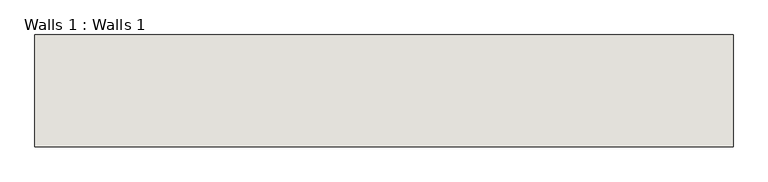
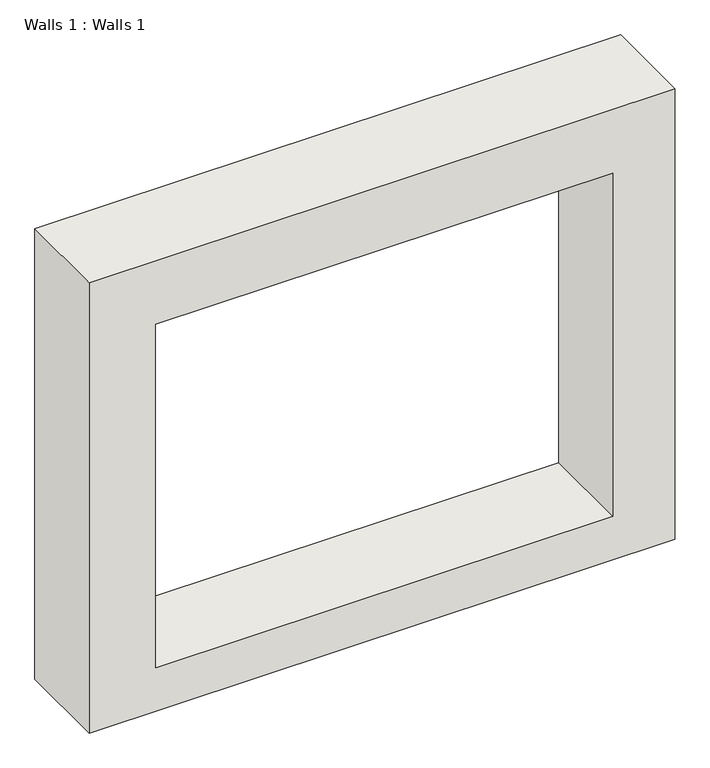
"""IFC4 building model written with IfcOpenShell, lengths in millimetres: wall geometry, Walls 1 : Walls 1."""

from ifc_helpers import new_model, si_unit, frame, origin, place, context, project, spatial, polyline, outline, extrude, source, transform, mapped, element, save


def walls_1_walls_1_6260b2a2(model_context):
    return source(origin(), model_context, "Body", "SweptSolid", [
        extrude(outline(polyline([(2334.2351899, -10249.5285704), (2334.2351899, -12154.5285704), (784.8351899, -12154.5285704), (784.8351899, -10249.5285704), (2334.2351899, -10249.5285704)]), holes=[polyline([(2114.55, -10450.9496792), (933.45, -10450.9496792), (933.45, -11936.8496792), (2114.55, -11936.8496792), (2114.55, -10450.9496792)])]), frame((0.0, -5876.9413939, 0.0), z_axis=(0.0, 1.0, 0.0), x_axis=(0.0, 0.0, 1.0)), (0.0, 0.0, 1.0), 304.8),
    ])


if __name__ == "__main__":
    model = new_model("IFC4")
    model_context = context("Model", 3, world=origin())
    ifc_project = project(units=[si_unit("LENGTHUNIT", "METRE", prefix="MILLI")], contexts=[model_context])
    site = spatial("IfcSite", under=ifc_project)
    building = spatial("IfcBuilding", under=site)
    placement = place(None, origin())
    walls_1_walls_1_shape = walls_1_walls_1_6260b2a2(model_context)
    element("IfcWall", 1, ObjectType="Walls 1 : Walls 1", at=placement, inside=building, context=model_context, shape_type="MappedRepresentation", body=[
        mapped(walls_1_walls_1_shape, transform((0.0, 0.0, 0.0), x_axis=(1.0, 0.0, 0.0), y_axis=(0.0, 1.0, 0.0), z_axis=(0.0, 0.0, 1.0))),
    ])
    save(model, "model.ifc")

# Revit data of these elements
# Element 1 (IfcWall, "Walls 1 : Walls 1")
#   Materials on its faces: "Default Wall"
# Materials
#   "Default Wall": colour RGB 80 80 80, transparency 0
